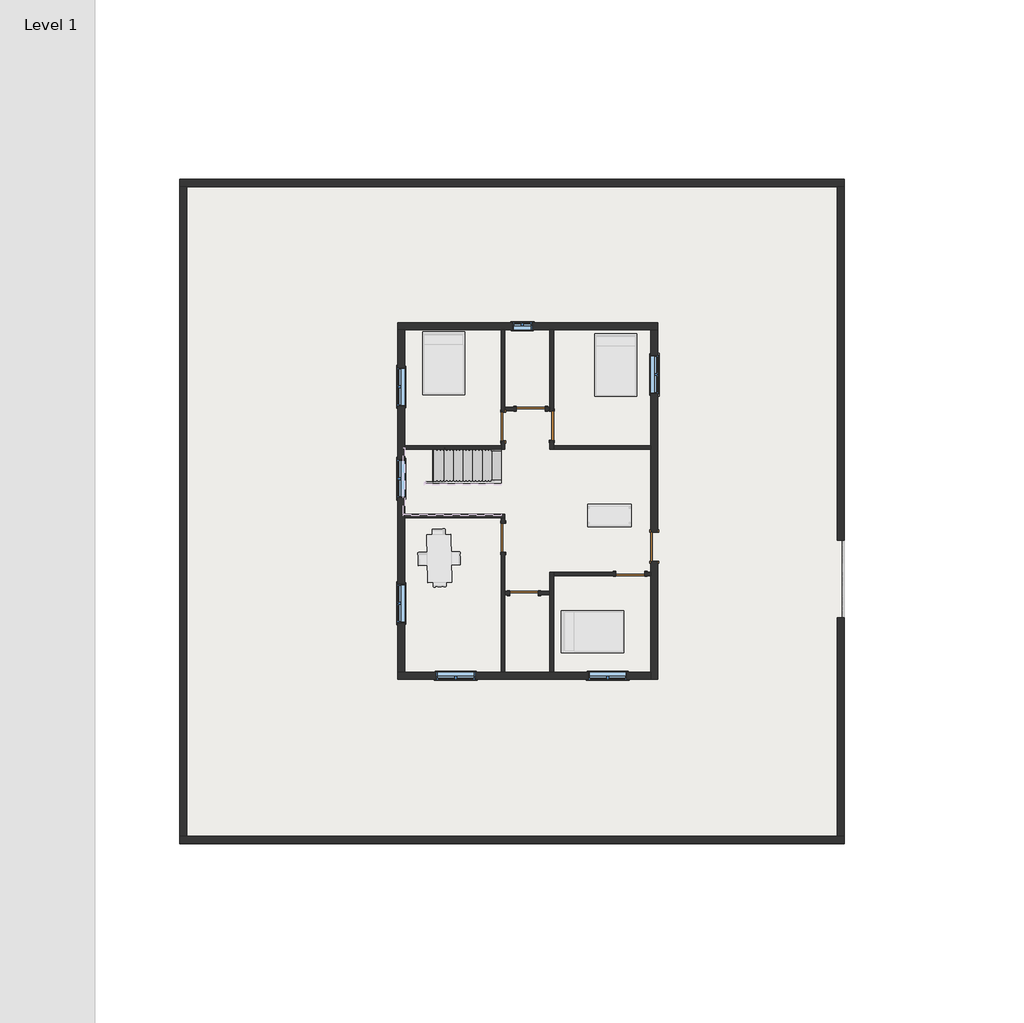
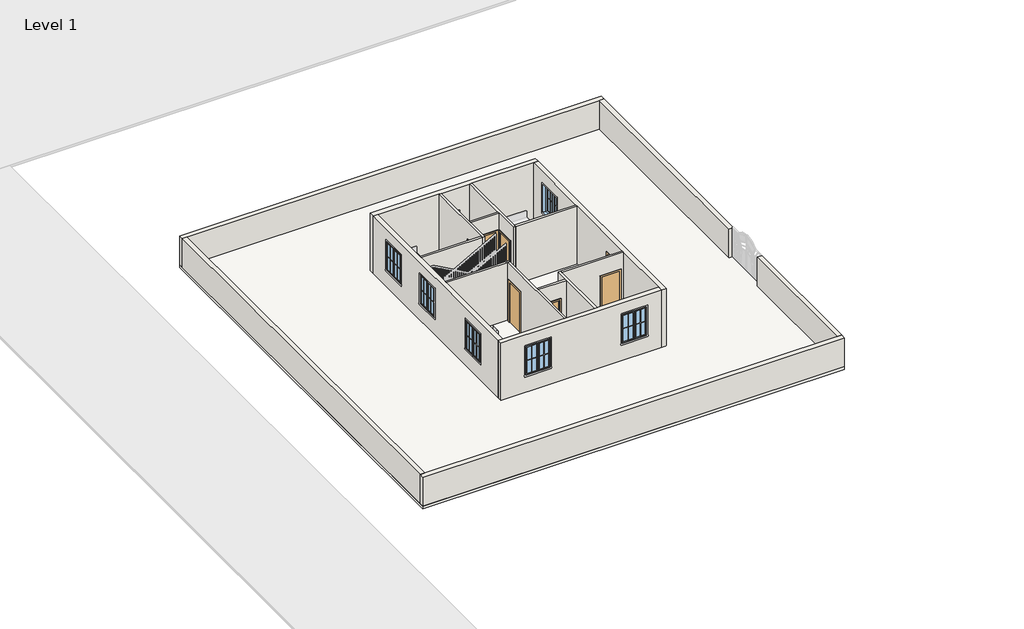
# One storey, part 1 of 3: 19 walls, 7 doors, 7 windows, 1 slab, 1 stair flight.
"""IFC4 building model written with IfcOpenShell, lengths in millimetres."""

from ifc_helpers import new_model, si_unit, frame, origin, origin_with_axes, place, context, project, spatial, polyline, outline, extrude, faceted_brep, transform, mapped, element, save
from components import door_e5f9f3c4, door_305aa2a5, door_a90ba1ad, stair_flight_dc0a5270, window_c417fced, window_8377141f

model = new_model("IFC4")

# Units and contexts
model_context = context("Model", 3, world=origin())
ifc_project = project(units=[si_unit("LENGTHUNIT", "METRE", prefix="MILLI")], contexts=[model_context])

# Site, building, storey
site = spatial("IfcSite", under=ifc_project)
building = spatial("IfcBuilding", under=site)
storey = spatial("IfcBuildingStorey", under=building, Name="Level 1", Elevation=0.0)

# Doors
placement = place(None, origin())
door_shape = door_e5f9f3c4(model_context)
element("IfcDoor", 1, ObjectType="Single-Flush : 36\" x 84\"", at=placement, inside=storey, context=model_context, shape_type="MappedRepresentation", body=[
    mapped(door_shape, transform((5226.05, 11245.85, 0.0), x_axis=(1.0, 0.0, 0.0), y_axis=(0.0, 1.0, 0.0), z_axis=(0.0, 0.0, 1.0))),
])
element("IfcDoor", 2, ObjectType="Single-Flush : 36\" x 84\"", at=placement, inside=storey, context=model_context, shape_type="MappedRepresentation", body=[
    mapped(door_shape, transform((5886.45, 10712.45, 0.0), x_axis=(0.0, -1.0, 0.0), y_axis=(1.0, 0.0, 0.0), z_axis=(0.0, 0.0, 1.0))),
])
door_2_shape = door_305aa2a5(model_context)
element("IfcDoor", 3, ObjectType="Single-Flush : 36\" x 84\"", at=placement, inside=storey, context=model_context, shape_type="MappedRepresentation", body=[
    mapped(door_2_shape, transform((4349.75, 10687.05, 0.0), x_axis=(0.0, -1.0, 0.0), y_axis=(1.0, 0.0, 0.0), z_axis=(0.0, 0.0, 1.0))),
])
element("IfcDoor", 4, ObjectType="Single-Flush : 36\" x 84\"", at=placement, inside=storey, context=model_context, shape_type="MappedRepresentation", body=[
    mapped(door_2_shape, transform((8369.3, 6026.15, 0.0), x_axis=(1.0, 0.0, 0.0), y_axis=(0.0, 1.0, 0.0), z_axis=(0.0, 0.0, 1.0))),
])
element("IfcDoor", 5, ObjectType="Single-Flush : 36\" x 84\"", at=placement, inside=storey, context=model_context, shape_type="MappedRepresentation", body=[
    mapped(door_2_shape, transform((5010.15, 5416.55, 0.0), x_axis=(-1.0, 0.0, 0.0), y_axis=(0.0, -1.0, 0.0), z_axis=(0.0, 0.0, 1.0))),
])
element("IfcDoor", 6, ObjectType="Single-Flush : 36\" x 84\"", at=placement, inside=storey, context=model_context, shape_type="MappedRepresentation", body=[
    mapped(door_2_shape, transform((4349.75, 7169.15, 0.0), x_axis=(0.0, -1.0, 0.0), y_axis=(1.0, 0.0, 0.0), z_axis=(0.0, 0.0, 1.0))),
])
door_3_shape = door_a90ba1ad(model_context)
element("IfcDoor", 7, ObjectType="Single-Flush : 36\" x 84\"", at=placement, inside=storey, context=model_context, shape_type="MappedRepresentation", body=[
    mapped(door_3_shape, transform((9131.3, 6889.75, 0.0), x_axis=(0.0, -1.0, 0.0), y_axis=(1.0, 0.0, 0.0), z_axis=(0.0, 0.0, 1.0))),
])

# Slab
element("IfcSlab", 8, ObjectType="Generic - 12\"", at=placement, inside=storey, context=model_context, shape_type="SweptSolid", body=[
    extrude(outline(polyline([(15146.2759659, 18504.2461341), (15146.2759659, -2501.5538659), (-5884.9240341, -2501.5538659), (-5884.9240341, 18504.2461341), (15146.2759659, 18504.2461341)])), frame((0.0, 0.0, -152.4), z_axis=(0.0, 0.0, 1.0), x_axis=(1.0, 0.0, 0.0)), (0.0, 0.0, 1.0), 152.4),
])

# Stair flight
stair_flight_shape = stair_flight_dc0a5270(model_context)
element("IfcStairFlight", 9, ObjectType="2\" Tread 1\" Nosing 1/4\" Riser", at=placement, inside=storey, context=model_context, shape_type="MappedRepresentation", body=[
    mapped(stair_flight_shape, transform((0.0, 0.0, 0.0), x_axis=(1.0, 0.0, 0.0), y_axis=(0.0, 1.0, 0.0), z_axis=(0.0, 0.0, 1.0))),
])

# Walls
element("IfcWall", 10, ObjectType="Generic - 5\"", at=placement, inside=storey, context=model_context, shape_type="Brep", body=[
    faceted_brep([(4292.6, 10229.85, 2133.6), (4292.6, 10229.85, 0.0), (4292.6, 10083.8, 0.0), (4292.6, 9969.5, 0.0), (4292.6, 9969.5, 3048.0), (4292.6, 10083.8, 3048.0), (4292.6, 13741.4, 3048.0), (4292.6, 13741.4, 0.0), (4292.6, 11144.25, 0.0), (4292.6, 11144.25, 2133.6), (4406.9, 9969.5, 0.0), (4406.9, 10229.85, 0.0), (4406.9, 10229.85, 2133.6), (4406.9, 11144.25, 2133.6), (4406.9, 11144.25, 0.0), (4406.9, 11188.7, 0.0), (4406.9, 11303.0, 0.0), (4406.9, 13741.4, 0.0), (4406.9, 13741.4, 3048.0), (4406.9, 11303.0, 3048.0), (4406.9, 11188.7, 3048.0), (4406.9, 9969.5, 3048.0)], [[[0, 1, 2, 3, 4, 5, 6, 7, 8, 9]], [[10, 11, 12, 13, 14, 15, 16, 17, 18, 19, 20, 21]], [[8, 7, 17, 16, 15, 14]], [[3, 2, 1, 11, 10]], [[6, 5, 4, 21, 20, 19, 18]], [[7, 6, 18, 17]], [[4, 3, 10, 21]], [[12, 11, 1, 0]], [[13, 12, 0, 9]], [[14, 13, 9, 8]]]),
])
element("IfcWall", 11, ObjectType="Generic - 5\"", at=placement, inside=storey, context=model_context, shape_type="SweptSolid", body=[
    extrude(outline(polyline([(1244.6, 10083.8), (4292.6, 10083.8), (4292.6, 9969.5), (1244.6, 9969.5), (1244.6, 10083.8)])), origin_with_axes(), (0.0, 0.0, 1.0), 3048.0),
])
element("IfcWall", 12, ObjectType="Generic - 5\"", at=placement, inside=storey, context=model_context, shape_type="SweptSolid", body=[
    extrude(outline(polyline([(2133.6, 5683.25), (0.0, 5683.25), (0.0, 5829.3), (3048.0, 5829.3), (3048.0, 4406.9), (0.0, 4406.9), (0.0, 4768.85), (2133.6, 4768.85), (2133.6, 5683.25)])), frame((0.0, 11188.7, 0.0), z_axis=(0.0, 1.0, 0.0), x_axis=(0.0, 0.0, 1.0)), (0.0, 0.0, 1.0), 114.3),
])
element("IfcWall", 13, ObjectType="Generic - 5\"", at=placement, inside=storey, context=model_context, shape_type="Brep", body=[
    faceted_brep([(5829.3, 10255.25, 2133.6), (5829.3, 10255.25, 0.0), (5829.3, 9969.5, 0.0), (5829.3, 9969.5, 3048.0), (5829.3, 11188.7, 3048.0), (5829.3, 11303.0, 3048.0), (5829.3, 13741.4, 3048.0), (5829.3, 13741.4, 0.0), (5829.3, 11303.0, 0.0), (5829.3, 11188.7, 0.0), (5829.3, 11169.65, 0.0), (5829.3, 11169.65, 2133.6), (5943.6, 9969.5, 0.0), (5943.6, 10083.8, 0.0), (5943.6, 10255.25, 0.0), (5943.6, 10255.25, 2133.6), (5943.6, 11169.65, 2133.6), (5943.6, 11169.65, 0.0), (5943.6, 13741.4, 0.0), (5943.6, 13741.4, 3048.0), (5943.6, 10083.8, 3048.0), (5943.6, 9969.5, 3048.0)], [[[0, 1, 2, 3, 4, 5, 6, 7, 8, 9, 10, 11]], [[12, 13, 14, 15, 16, 17, 18, 19, 20, 21]], [[2, 1, 14, 13, 12]], [[10, 9, 8, 7, 18, 17]], [[6, 5, 4, 3, 21, 20, 19]], [[7, 6, 19, 18]], [[3, 2, 12, 21]], [[15, 14, 1, 0]], [[16, 15, 0, 11]], [[17, 16, 11, 10]]]),
])
element("IfcWall", 14, ObjectType="Generic - 5\"", at=placement, inside=storey, context=model_context, shape_type="SweptSolid", body=[
    extrude(outline(polyline([(9017.0, 9969.5), (5943.6, 9969.5), (5943.6, 10083.8), (9017.0, 10083.8), (9017.0, 9969.5)])), origin_with_axes(), (0.0, 0.0, 1.0), 3048.0),
])
element("IfcWall", 15, ObjectType="Generic - 5\"", at=placement, inside=storey, context=model_context, shape_type="Brep", body=[
    faceted_brep([(1244.6, 7797.8, 0.0), (4292.6, 7797.8, 0.0), (4406.9, 7797.8, 0.0), (4406.9, 7797.8, 3048.0), (4292.6, 7797.8, 3048.0), (1244.6, 7797.8, 3048.0), (1244.6, 7912.1, 0.0), (1244.6, 7912.1, 3048.0), (4406.9, 7912.1, 3048.0), (4406.9, 7912.1, 0.0)], [[[0, 1, 2, 3, 4, 5]], [[6, 7, 8, 9]], [[2, 1, 0, 6, 9]], [[5, 4, 3, 8, 7]], [[0, 5, 7, 6]], [[3, 2, 9, 8]]]),
])
element("IfcWall", 16, ObjectType="Generic - 5\"", at=placement, inside=storey, context=model_context, shape_type="Brep", body=[
    faceted_brep([(4292.6, 6711.95, 2133.6), (4292.6, 6711.95, 0.0), (4292.6, 2921.0, 0.0), (4292.6, 2921.0, 3048.0), (4292.6, 7797.8, 3048.0), (4292.6, 7797.8, 0.0), (4292.6, 7626.35, 0.0), (4292.6, 7626.35, 2133.6), (4406.9, 2921.0, 0.0), (4406.9, 5359.4, 0.0), (4406.9, 5473.7, 0.0), (4406.9, 6711.95, 0.0), (4406.9, 6711.95, 2133.6), (4406.9, 7626.35, 2133.6), (4406.9, 7626.35, 0.0), (4406.9, 7797.8, 0.0), (4406.9, 7797.8, 3048.0), (4406.9, 5473.7, 3048.0), (4406.9, 5359.4, 3048.0), (4406.9, 2921.0, 3048.0)], [[[0, 1, 2, 3, 4, 5, 6, 7]], [[8, 9, 10, 11, 12, 13, 14, 15, 16, 17, 18, 19]], [[6, 5, 15, 14]], [[2, 1, 11, 10, 9, 8]], [[4, 3, 19, 18, 17, 16]], [[5, 4, 16, 15]], [[3, 2, 8, 19]], [[12, 11, 1, 0]], [[13, 12, 0, 7]], [[14, 13, 7, 6]]]),
])
element("IfcWall", 17, ObjectType="Generic - 5\"", at=placement, inside=storey, context=model_context, shape_type="SweptSolid", body=[
    extrude(outline(polyline([(0.0, 4406.9), (0.0, 4552.95), (2133.6, 4552.95), (2133.6, 5467.35), (0.0, 5467.35), (0.0, 5829.3), (3048.0, 5829.3), (3048.0, 4406.9), (0.0, 4406.9)])), frame((0.0, 5359.4, 0.0), z_axis=(0.0, 1.0, 0.0), x_axis=(0.0, 0.0, 1.0)), (0.0, 0.0, 1.0), 114.3),
])
element("IfcWall", 18, ObjectType="Generic - 5\"", at=placement, inside=storey, context=model_context, shape_type="Brep", body=[
    faceted_brep([(5943.6, 2921.0, 0.0), (5943.6, 5969.0, 0.0), (5943.6, 6083.3, 0.0), (5943.6, 6083.3, 3048.0), (5943.6, 5969.0, 3048.0), (5943.6, 2921.0, 3048.0), (5829.3, 2921.0, 0.0), (5829.3, 2921.0, 3048.0), (5829.3, 5359.4, 3048.0), (5829.3, 5473.7, 3048.0), (5829.3, 6083.3, 3048.0), (5829.3, 6083.3, 0.0), (5829.3, 5473.7, 0.0), (5829.3, 5359.4, 0.0)], [[[0, 1, 2, 3, 4, 5]], [[6, 7, 8, 9, 10, 11, 12, 13]], [[2, 1, 0, 6, 13, 12, 11]], [[5, 4, 3, 10, 9, 8, 7]], [[0, 5, 7, 6]], [[3, 2, 11, 10]]]),
])
element("IfcWall", 19, ObjectType="Generic - 5\"", at=placement, inside=storey, context=model_context, shape_type="SweptSolid", body=[
    extrude(outline(polyline([(2133.6, 8826.5), (0.0, 8826.5), (0.0, 9017.0), (3048.0, 9017.0), (3048.0, 5943.6), (0.0, 5943.6), (0.0, 7912.1), (2133.6, 7912.1), (2133.6, 8826.5)])), frame((0.0, 5969.0, 0.0), z_axis=(0.0, 1.0, 0.0), x_axis=(0.0, 0.0, 1.0)), (0.0, 0.0, 1.0), 114.3),
])
element("IfcWall", 20, ObjectType="Generic - 8\"", at=placement, inside=storey, context=model_context, shape_type="Brep", body=[
    faceted_brep([(1016.0, 13741.4, 0.0), (1244.6, 13741.4, 0.0), (4292.6, 13741.4, 0.0), (4406.9, 13741.4, 0.0), (5829.3, 13741.4, 0.0), (5943.6, 13741.4, 0.0), (9017.0, 13741.4, 0.0), (9245.6, 13741.4, 0.0), (9245.6, 13741.4, 3048.0), (9017.0, 13741.4, 3048.0), (5943.6, 13741.4, 3048.0), (5829.3, 13741.4, 3048.0), (4406.9, 13741.4, 3048.0), (4292.6, 13741.4, 3048.0), (1244.6, 13741.4, 3048.0), (1016.0, 13741.4, 3048.0), (5264.15, 13741.4, 1828.8), (5264.15, 13741.4, 914.4), (4654.55, 13741.4, 914.4), (4654.55, 13741.4, 1828.8), (1016.0, 13970.0, 0.0), (1016.0, 13970.0, 3048.0), (9245.6, 13970.0, 3048.0), (9245.6, 13970.0, 0.0), (5264.15, 13970.0, 1828.8), (4654.55, 13970.0, 1828.8), (4654.55, 13970.0, 914.4), (5264.15, 13970.0, 914.4)], [[[0, 1, 2, 3, 4, 5, 6, 7, 8, 9, 10, 11, 12, 13, 14, 15], [16, 17, 18, 19]], [[20, 21, 22, 23], [24, 25, 26, 27]], [[7, 6, 5, 4, 3, 2, 1, 0, 20, 23]], [[8, 7, 23, 22]], [[0, 15, 21, 20]], [[17, 16, 24, 27]], [[18, 17, 27, 26]], [[19, 18, 26, 25]], [[16, 19, 25, 24]], [[15, 14, 13, 12, 11, 10, 9, 8, 22, 21]]]),
])
element("IfcWall", 21, ObjectType="Generic - 8\"", at=placement, inside=storey, context=model_context, shape_type="Brep", body=[
    faceted_brep([(9017.0, 6432.55, 2133.6), (9017.0, 6432.55, 0.0), (9017.0, 6083.3, 0.0), (9017.0, 5969.0, 0.0), (9017.0, 2921.0, 0.0), (9017.0, 2692.4, 0.0), (9017.0, 2692.4, 3048.0), (9017.0, 2921.0, 3048.0), (9017.0, 5969.0, 3048.0), (9017.0, 6083.3, 3048.0), (9017.0, 9969.5, 3048.0), (9017.0, 10083.8, 3048.0), (9017.0, 13741.4, 3048.0), (9017.0, 13741.4, 0.0), (9017.0, 10083.8, 0.0), (9017.0, 9969.5, 0.0), (9017.0, 7346.95, 0.0), (9017.0, 7346.95, 2133.6), (9017.0, 11722.1, 2438.4), (9017.0, 11722.1, 914.4), (9017.0, 12941.3, 914.4), (9017.0, 12941.3, 2438.4), (9245.6, 2692.4, 0.0), (9245.6, 6432.55, 0.0), (9245.6, 6432.55, 2133.6), (9245.6, 7346.95, 2133.6), (9245.6, 7346.95, 0.0), (9245.6, 13741.4, 0.0), (9245.6, 13741.4, 3048.0), (9245.6, 2692.4, 3048.0), (9245.6, 11722.1, 2438.4), (9245.6, 12941.3, 2438.4), (9245.6, 12941.3, 914.4), (9245.6, 11722.1, 914.4)], [[[0, 1, 2, 3, 4, 5, 6, 7, 8, 9, 10, 11, 12, 13, 14, 15, 16, 17], [18, 19, 20, 21]], [[22, 23, 24, 25, 26, 27, 28, 29], [30, 31, 32, 33]], [[5, 4, 3, 2, 1, 23, 22]], [[16, 15, 14, 13, 27, 26]], [[13, 12, 28, 27]], [[6, 5, 22, 29]], [[24, 23, 1, 0]], [[25, 24, 0, 17]], [[26, 25, 17, 16]], [[19, 18, 30, 33]], [[20, 19, 33, 32]], [[21, 20, 32, 31]], [[18, 21, 31, 30]], [[12, 11, 10, 9, 8, 7, 6, 29, 28]]]),
])
element("IfcWall", 22, ObjectType="Generic - 8\"", at=placement, inside=storey, context=model_context, shape_type="Brep", body=[
    faceted_brep([(9017.0, 2921.0, 0.0), (5943.6, 2921.0, 0.0), (5829.3, 2921.0, 0.0), (4406.9, 2921.0, 0.0), (4292.6, 2921.0, 0.0), (1244.6, 2921.0, 0.0), (1016.0, 2921.0, 0.0), (1016.0, 2921.0, 3048.0), (1244.6, 2921.0, 3048.0), (4292.6, 2921.0, 3048.0), (4406.9, 2921.0, 3048.0), (5829.3, 2921.0, 3048.0), (5943.6, 2921.0, 3048.0), (9017.0, 2921.0, 3048.0), (7048.5, 2921.0, 2438.4), (7048.5, 2921.0, 914.4), (8267.7, 2921.0, 914.4), (8267.7, 2921.0, 2438.4), (2241.55, 2921.0, 2438.4), (2241.55, 2921.0, 914.4), (3460.75, 2921.0, 914.4), (3460.75, 2921.0, 2438.4), (9017.0, 2692.4, 0.0), (9017.0, 2692.4, 3048.0), (1016.0, 2692.4, 3048.0), (1016.0, 2692.4, 0.0), (7048.5, 2692.4, 2438.4), (8267.7, 2692.4, 2438.4), (8267.7, 2692.4, 914.4), (7048.5, 2692.4, 914.4), (2241.55, 2692.4, 2438.4), (3460.75, 2692.4, 2438.4), (3460.75, 2692.4, 914.4), (2241.55, 2692.4, 914.4)], [[[0, 1, 2, 3, 4, 5, 6, 7, 8, 9, 10, 11, 12, 13], [14, 15, 16, 17], [18, 19, 20, 21]], [[22, 23, 24, 25], [26, 27, 28, 29], [30, 31, 32, 33]], [[6, 5, 4, 3, 2, 1, 0, 22, 25]], [[0, 13, 23, 22]], [[7, 6, 25, 24]], [[15, 14, 26, 29]], [[16, 15, 29, 28]], [[17, 16, 28, 27]], [[14, 17, 27, 26]], [[19, 18, 30, 33]], [[20, 19, 33, 32]], [[21, 20, 32, 31]], [[18, 21, 31, 30]], [[13, 12, 11, 10, 9, 8, 7, 24, 23]]]),
])
element("IfcWall", 23, ObjectType="Generic - 8\"", at=placement, inside=storey, context=model_context, shape_type="Brep", body=[
    faceted_brep([(1244.6, 2921.0, 0.0), (1244.6, 7797.8, 0.0), (1244.6, 7912.1, 0.0), (1244.6, 9969.5, 0.0), (1244.6, 10083.8, 0.0), (1244.6, 13741.4, 0.0), (1244.6, 13741.4, 3048.0), (1244.6, 10083.8, 3048.0), (1244.6, 9969.5, 3048.0), (1244.6, 7912.1, 3048.0), (1244.6, 7797.8, 3048.0), (1244.6, 2921.0, 3048.0), (1244.6, 5702.3, 2438.4), (1244.6, 5702.3, 914.4), (1244.6, 4483.1, 914.4), (1244.6, 4483.1, 2438.4), (1244.6, 9645.65, 2438.4), (1244.6, 9645.65, 914.4), (1244.6, 8426.45, 914.4), (1244.6, 8426.45, 2438.4), (1244.6, 12550.775, 2438.4), (1244.6, 12550.775, 914.4), (1244.6, 11331.575, 914.4), (1244.6, 11331.575, 2438.4), (1016.0, 2921.0, 0.0), (1016.0, 2921.0, 3048.0), (1016.0, 13741.4, 3048.0), (1016.0, 13741.4, 0.0), (1016.0, 5702.3, 2438.4), (1016.0, 4483.1, 2438.4), (1016.0, 4483.1, 914.4), (1016.0, 5702.3, 914.4), (1016.0, 9645.65, 2438.4), (1016.0, 8426.45, 2438.4), (1016.0, 8426.45, 914.4), (1016.0, 9645.65, 914.4), (1016.0, 12550.775, 2438.4), (1016.0, 11331.575, 2438.4), (1016.0, 11331.575, 914.4), (1016.0, 12550.775, 914.4)], [[[0, 1, 2, 3, 4, 5, 6, 7, 8, 9, 10, 11], [12, 13, 14, 15], [16, 17, 18, 19], [20, 21, 22, 23]], [[24, 25, 26, 27], [28, 29, 30, 31], [32, 33, 34, 35], [36, 37, 38, 39]], [[5, 4, 3, 2, 1, 0, 24, 27]], [[6, 5, 27, 26]], [[0, 11, 25, 24]], [[13, 12, 28, 31]], [[14, 13, 31, 30]], [[15, 14, 30, 29]], [[12, 15, 29, 28]], [[17, 16, 32, 35]], [[18, 17, 35, 34]], [[19, 18, 34, 33]], [[16, 19, 33, 32]], [[21, 20, 36, 39]], [[22, 21, 39, 38]], [[23, 22, 38, 37]], [[20, 23, 37, 36]], [[11, 10, 9, 8, 7, 6, 26, 25]]]),
])
element("IfcWall", 24, ObjectType="Generic - 8\"", at=placement, inside=storey, context=model_context, shape_type="Brep", body=[
    faceted_brep([(-5884.9240341, 18275.6461341, 0.0), (-5656.3240341, 18275.6461341, 0.0), (14917.6759659, 18275.6461341, 0.0), (15146.2759659, 18275.6461341, 0.0), (15146.2759659, 18275.6461341, 1524.0), (14917.6759659, 18275.6461341, 1524.0), (-5656.3240341, 18275.6461341, 1524.0), (-5884.9240341, 18275.6461341, 1524.0), (-5884.9240341, 18504.2461341, 0.0), (-5884.9240341, 18504.2461341, 1524.0), (15146.2759659, 18504.2461341, 1524.0), (15146.2759659, 18504.2461341, 0.0)], [[[0, 1, 2, 3, 4, 5, 6, 7]], [[8, 9, 10, 11]], [[3, 2, 1, 0, 8, 11]], [[7, 6, 5, 4, 10, 9]], [[4, 3, 11, 10]], [[0, 7, 9, 8]]]),
])
element("IfcWall", 25, ObjectType="Generic - 8\"", at=placement, inside=storey, context=model_context, shape_type="SweptSolid", body=[
    extrude(outline(polyline([(14917.6759659, 7086.9461341), (14917.6759659, 18275.6461341), (15146.2759659, 18275.6461341), (15146.2759659, 7086.9461341), (14917.6759659, 7086.9461341)])), origin_with_axes(), (0.0, 0.0, 1.0), 1524.0),
])
element("IfcWall", 26, ObjectType="Generic - 8\"", at=placement, inside=storey, context=model_context, shape_type="Brep", body=[
    faceted_brep([(15138.8257267, -2272.9538659, 0.0), (14910.2257267, -2272.9538659, 0.0), (-5656.3240341, -2272.9538659, 0.0), (-5884.9240341, -2272.9538659, 0.0), (-5884.9240341, -2272.9538659, 1524.0), (-5656.3240341, -2272.9538659, 1524.0), (14910.2257267, -2272.9538659, 1524.0), (15138.8257267, -2272.9538659, 1524.0), (15138.8257267, -2501.5538659, 0.0), (15138.8257267, -2501.5538659, 1524.0), (-5884.9240341, -2501.5538659, 1524.0), (-5884.9240341, -2501.5538659, 0.0)], [[[0, 1, 2, 3, 4, 5, 6, 7]], [[8, 9, 10, 11]], [[3, 2, 1, 0, 8, 11]], [[7, 6, 5, 4, 10, 9]], [[4, 3, 11, 10]], [[0, 7, 9, 8]]]),
])
element("IfcWall", 27, ObjectType="Generic - 8\"", at=placement, inside=storey, context=model_context, shape_type="SweptSolid", body=[
    extrude(outline(polyline([(-5656.3240341, 18275.6461341), (-5656.3240341, -2272.9538659), (-5884.9240341, -2272.9538659), (-5884.9240341, 18275.6461341), (-5656.3240341, 18275.6461341)])), origin_with_axes(), (0.0, 0.0, 1.0), 1524.0),
])
element("IfcWall", 28, ObjectType="Generic - 8\"", at=placement, inside=storey, context=model_context, shape_type="SweptSolid", body=[
    extrude(outline(polyline([(14910.2257267, -2272.9538659), (14910.2257267, 4631.8639368), (15138.8257267, 4631.8639368), (15138.8257267, -2272.9538659), (14910.2257267, -2272.9538659)])), origin_with_axes(), (0.0, 0.0, 1.0), 1524.0),
])

# Windows
window_shape = window_c417fced(model_context)
element("IfcWindow", 29, ObjectType="Window-Casement-Double : 24\" x 36\"", at=placement, inside=storey, context=model_context, shape_type="MappedRepresentation", body=[
    mapped(window_shape, transform((4959.35, 13855.7, 0.0), x_axis=(1.0, 0.0, 0.0), y_axis=(0.0, 1.0, 0.0), z_axis=(0.0, 0.0, 1.0))),
])
window_2_shape = window_8377141f(model_context)
element("IfcWindow", 30, ObjectType="Window-Casement-Double : 48\" x 60\"", at=placement, inside=storey, context=model_context, shape_type="MappedRepresentation", body=[
    mapped(window_2_shape, transform((7658.1, 2806.7, 0.0), x_axis=(-1.0, 0.0, 0.0), y_axis=(0.0, -1.0, 0.0), z_axis=(0.0, 0.0, 1.0))),
])
element("IfcWindow", 31, ObjectType="Window-Casement-Double : 48\" x 60\"", at=placement, inside=storey, context=model_context, shape_type="MappedRepresentation", body=[
    mapped(window_2_shape, transform((2851.15, 2806.7, 0.0), x_axis=(-1.0, 0.0, 0.0), y_axis=(0.0, -1.0, 0.0), z_axis=(0.0, 0.0, 1.0))),
])
element("IfcWindow", 32, ObjectType="Window-Casement-Double : 48\" x 60\"", at=placement, inside=storey, context=model_context, shape_type="MappedRepresentation", body=[
    mapped(window_2_shape, transform((1130.3, 5092.7, 0.0), x_axis=(0.0, 1.0, 0.0), y_axis=(-1.0, 0.0, 0.0), z_axis=(0.0, 0.0, 1.0))),
])
element("IfcWindow", 33, ObjectType="Window-Casement-Double : 48\" x 60\"", at=placement, inside=storey, context=model_context, shape_type="MappedRepresentation", body=[
    mapped(window_2_shape, transform((1130.3, 9036.05, 0.0), x_axis=(0.0, 1.0, 0.0), y_axis=(-1.0, 0.0, 0.0), z_axis=(0.0, 0.0, 1.0))),
])
element("IfcWindow", 34, ObjectType="Window-Casement-Double : 48\" x 60\"", at=placement, inside=storey, context=model_context, shape_type="MappedRepresentation", body=[
    mapped(window_2_shape, transform((1130.3, 11941.175, 0.0), x_axis=(0.0, 1.0, 0.0), y_axis=(-1.0, 0.0, 0.0), z_axis=(0.0, 0.0, 1.0))),
])
element("IfcWindow", 35, ObjectType="Window-Casement-Double : 48\" x 60\"", at=placement, inside=storey, context=model_context, shape_type="MappedRepresentation", body=[
    mapped(window_2_shape, transform((9131.3, 12331.7, 0.0), x_axis=(0.0, -1.0, 0.0), y_axis=(1.0, 0.0, 0.0), z_axis=(0.0, 0.0, 1.0))),
])

save(model, "model.ifc")

# Revit data of these elements
# Type "Single-Flush : 36\" x 84\""
#   Type Mark = "1"
#   Construction Type Id = "MDOOR"
#   Assembly Code = "C1020"
#   Analytic Construction = "Metal"
#   Thickness = 0' - 2"
#   Heat Transfer Coefficient (U) = 0.651978 BTU/(h·ft²·°F)
#   Height = 7' - 0"
#   Trim Projection Ext = 0' - 1"
#   Trim Projection Int = 0' - 1"
#   Trim Width = 0' - 3"
#   Width = 3' - 0"
#   Define Thermal Properties by = 1
#   Define Thermal Properties by = 1
#   Door Material = Door - Panel
#   Frame Material = Door - Frame
#   Visual Light Transmittance = 0
#   Solar Heat Gain Coefficient = 0
#   Function = (empty or 0)
#   Wall Closure = (empty or 0)
# Type "Generic - 12\""
#   Assembly Code = "B1010"
#   Function = 0
#   Layers, outside or top first: 0' - 6" no material (function 1)
# Type "Generic - 5\""
#   Assembly Code = "B2010"
#   Layers, outside or top first: 0' - 4 1/2" no material (function 1)
# Type "Generic - 8\""
#   Assembly Code = "B2010"
#   Layers, outside or top first: 0' - 9" no material (function 1)
# Type "Window-Casement-Double : 24\" x 36\""
#   Type Mark = "14"
#   Fire Rating = "0.5h"
#   Assembly Code = "B2020100"
#   Analytic Construction = "Double glazing - domestic"
#   Frame Extension [instance default] = 0' - 0 1/4"
#   Window Inset [instance default] = 0' - 0"
#   Wall Thickness [instance default] = 0' - 6"
#   Interior Wall Closure [instance default] = 0' - 2 1/4"
#   Half Width = 1' - 0"
#   Visual Light Transmittance = 0.81
#   Thermal Resistance (R) = 1.8146 (h·ft²·°F)/BTU
#   Solar Heat Gain Coefficient = 0.76
#   Rough Width = 2' - 0 1/2"
#   Rough Height = 3' - 0 1/2"
#   Height = 3' - 0"
#   Heat Transfer Coefficient (U) = 0.5511 BTU/(h·ft²·°F)
#   Exterior Wall Closure [instance default] = 0' - 1 1/4"
#   Extension Jamb [instance default] = 0' - 2 1/4"
#   Default Sill Height = 3' - 0"
#   Width = 2' - 0"
#   Define Thermal Properties by = 0
#   Muntin Visibility = yes
#   Interior Trim Visibility [instance default] = yes
#   Exterior Trim Visibility [instance default] = yes
#   Extension Jamb Visibility [instance default] = yes
#   Interior Trim Material = Wood - Stained
#   Muntin Pattern = Muntin Pattern_2x2 : Muntin Pattern_2x2
#   Interior Trim = Trim-Window-Interior-Flat : Picture Frame
#   Interior Frame Material = Wood - Stained
#   Glass Panel Material = Glass
#   Exterior Trim Material = Clad - White
#   Exterior Trim = Trim-Window-Exterior-Flat : with Sill
#   Exterior Frame Material = Clad - White
#   Wall Closure = (empty or 0)
# Type "Window-Casement-Double : 48\" x 60\""
#   Type Mark = "17"
#   Fire Rating = "0.5h"
#   Assembly Code = "B2020100"
#   Analytic Construction = "Double glazing - domestic"
#   Frame Extension [instance default] = 0' - 0 1/4"
#   Window Inset [instance default] = 0' - 0"
#   Wall Thickness [instance default] = 0' - 6"
#   Interior Wall Closure [instance default] = 0' - 2 1/4"
#   Half Width = 2' - 0"
#   Visual Light Transmittance = 0.81
#   Thermal Resistance (R) = 1.8146 (h·ft²·°F)/BTU
#   Solar Heat Gain Coefficient = 0.76
#   Rough Width = 4' - 0 1/2"
#   Rough Height = 5' - 0 1/2"
#   Height = 5' - 0"
#   Heat Transfer Coefficient (U) = 0.5511 BTU/(h·ft²·°F)
#   Exterior Wall Closure [instance default] = 0' - 1 1/4"
#   Extension Jamb [instance default] = 0' - 2 1/4"
#   Default Sill Height = 3' - 0"
#   Width = 4' - 0"
#   Define Thermal Properties by = 0
#   Muntin Visibility = yes
#   Interior Trim Visibility [instance default] = yes
#   Exterior Trim Visibility [instance default] = yes
#   Extension Jamb Visibility [instance default] = yes
#   Interior Trim Material = Wood - Stained
#   Muntin Pattern = Muntin Pattern_2x2 : Muntin Pattern_2x2
#   Interior Trim = Trim-Window-Interior-Flat : Picture Frame
#   Interior Frame Material = Wood - Stained
#   Glass Panel Material = Glass
#   Exterior Trim Material = Clad - White
#   Exterior Trim = Trim-Window-Exterior-Flat : with Sill
#   Exterior Frame Material = Clad - White
#   Wall Closure = (empty or 0)
# Elements 1, 2, 3, 4, 5, 6, 7 (IfcDoor, "Single-Flush : 36\" x 84\"")
#   Phase Created = New Construction
#   Materials on its faces: "Door - Frame", "Door - Panel"
# Element 8 (IfcSlab, "Generic - 12\"")
#   Height Offset From Level = 0' - 0"
#   Phase Created = New Construction
#   Materials on its faces: "Flor_Branco", "Default Floor", "Wood Planks"
# Element 9 (IfcStairFlight, "2\" Tread 1\" Nosing 1/4\" Riser")
#   Phase Created = New Construction
# Elements 10, 11, 12, 13, 14, 15, 16, 17, 18, 19 (IfcWall, "Generic - 5\"")
#   Top Offset = 0' - 0"
#   Base Offset = 0' - 0"
#   wall height = 10' - 0"
#   Phase Created = New Construction
#   Base Constraint = Level 1
#   Top Constraint = Level 2
#   Materials on its faces: "Default Wall"
# Elements 20, 21, 22, 23 (IfcWall, "Generic - 8\"")
#   Top Offset = 0' - 0"
#   Base Offset = 0' - 0"
#   Unconnected Height = 10' - 0"
#   wall height = 10' - 0"
#   Phase Created = New Construction
#   Base Constraint = Level 1
#   Materials on its faces: "Default Wall", "Sash"
# Elements 24, 26 (IfcWall, "Generic - 8\"")
#   Top Offset = 0' - 0"
#   Base Offset = 0' - 0"
#   Unconnected Height = 5' - 0"
#   wall height = 5' - 0"
#   Phase Created = New Construction
#   Base Constraint = Level 1
#   Materials on its faces: "Flor_Branco", "Wood Planks", "Default Wall", "Oak Flooring"
# Elements 25, 27 (IfcWall, "Generic - 8\"")
#   Top Offset = 0' - 0"
#   Base Offset = 0' - 0"
#   Unconnected Height = 5' - 0"
#   wall height = 5' - 0"
#   Phase Created = New Construction
#   Base Constraint = Level 1
#   Materials on its faces: "Default Wall", "Wood Planks", "Flor_Branco", "Oak Flooring"
# Element 28 (IfcWall, "Generic - 8\"")
#   Top Offset = 0' - 0"
#   Base Offset = 0' - 0"
#   Unconnected Height = 5' - 0"
#   wall height = 5' - 0"
#   Phase Created = New Construction
#   Base Constraint = Level 1
#   Materials on its faces: "Default Wall", "Oak Flooring", "Flor_Branco"
# Element 29 (IfcWindow, "Window-Casement-Double : 24\" x 36\"")
#   Mark = "7"
#   Window Inset = 0' - 0"
#   Interior Wall Closure = 0' - 2 1/4"
#   Frame Extension = 0' - 0 1/4"
#   Exterior Wall Closure = 0' - 1 1/4"
#   Interior Trim Visibility = yes
#   Exterior Trim Visibility = yes
#   Phase Created = New Construction
#   Materials on its faces: "Wood - Stained", "Glass", "Clad - White"
# Element 30 (IfcWindow, "Window-Casement-Double : 48\" x 60\"")
#   Mark = "1"
#   Window Inset = 0' - 0"
#   Interior Wall Closure = 0' - 2 1/4"
#   Frame Extension = 0' - 0 1/4"
#   Exterior Wall Closure = 0' - 1 1/4"
#   Interior Trim Visibility = yes
#   Exterior Trim Visibility = yes
#   Phase Created = New Construction
#   Materials on its faces: "Wood - Stained", "Glass", "Clad - White"
# Element 31 (IfcWindow, "Window-Casement-Double : 48\" x 60\"")
#   Mark = "2"
#   Window Inset = 0' - 0"
#   Interior Wall Closure = 0' - 2 1/4"
#   Frame Extension = 0' - 0 1/4"
#   Exterior Wall Closure = 0' - 1 1/4"
#   Interior Trim Visibility = yes
#   Exterior Trim Visibility = yes
#   Phase Created = New Construction
#   Materials on its faces: "Wood - Stained", "Glass", "Clad - White"
# Element 32 (IfcWindow, "Window-Casement-Double : 48\" x 60\"")
#   Mark = "3"
#   Window Inset = 0' - 0"
#   Interior Wall Closure = 0' - 2 1/4"
#   Frame Extension = 0' - 0 1/4"
#   Exterior Wall Closure = 0' - 1 1/4"
#   Interior Trim Visibility = yes
#   Exterior Trim Visibility = yes
#   Phase Created = New Construction
#   Materials on its faces: "Wood - Stained", "Glass", "Clad - White"
# Element 33 (IfcWindow, "Window-Casement-Double : 48\" x 60\"")
#   Mark = "4"
#   Window Inset = 0' - 0"
#   Interior Wall Closure = 0' - 2 1/4"
#   Frame Extension = 0' - 0 1/4"
#   Exterior Wall Closure = 0' - 1 1/4"
#   Interior Trim Visibility = yes
#   Exterior Trim Visibility = yes
#   Phase Created = New Construction
#   Materials on its faces: "Wood - Stained", "Glass", "Clad - White"
# Element 34 (IfcWindow, "Window-Casement-Double : 48\" x 60\"")
#   Mark = "5"
#   Window Inset = 0' - 0"
#   Interior Wall Closure = 0' - 2 1/4"
#   Frame Extension = 0' - 0 1/4"
#   Exterior Wall Closure = 0' - 1 1/4"
#   Interior Trim Visibility = yes
#   Exterior Trim Visibility = yes
#   Phase Created = New Construction
#   Materials on its faces: "Wood - Stained", "Glass", "Clad - White"
# Element 35 (IfcWindow, "Window-Casement-Double : 48\" x 60\"")
#   Mark = "6"
#   Window Inset = 0' - 0"
#   Interior Wall Closure = 0' - 2 1/4"
#   Frame Extension = 0' - 0 1/4"
#   Exterior Wall Closure = 0' - 1 1/4"
#   Interior Trim Visibility = yes
#   Exterior Trim Visibility = yes
#   Phase Created = New Construction
#   Materials on its faces: "Wood - Stained", "Glass", "Clad - White"
# Materials
#   "Door - Panel": class "Wood", colour RGB 210 159 95, transparency 0, Cost = 0
#   "Door - Frame": colour RGB 118 70 51, transparency 0, Cost = 0
#   "Wood - Stained": class "Wood", colour RGB 224 178 126, transparency 0, Cost = 0
#   "Glass": class "Glass", colour RGB 0 128 192, transparency 0.75, Description = "Soda Lime Glass", Cost = 0
#   "Clad - White": class "Wood", colour RGB 242 242 238, transparency 0, Cost = 0
#   "Flor_Branco": class "Paint", colour RGB 255 255 255, transparency 0
#   "Default Floor": colour RGB 128 128 128, transparency 0, Cost = 0
#   "Wood Planks": class "Wood", colour RGB 193 160 115, transparency 0, Description = "Physical material.", Cost = 0
#   "Default Wall": colour RGB 128 128 128, transparency 0, Cost = 0
#   "Sash": class "Wood", colour RGB 224 178 126, transparency 0, Cost = 0
#   "Oak Flooring": class "Wood", colour RGB 216 169 114, transparency 0, Description = "Quercus Rubra", Cost = 0
